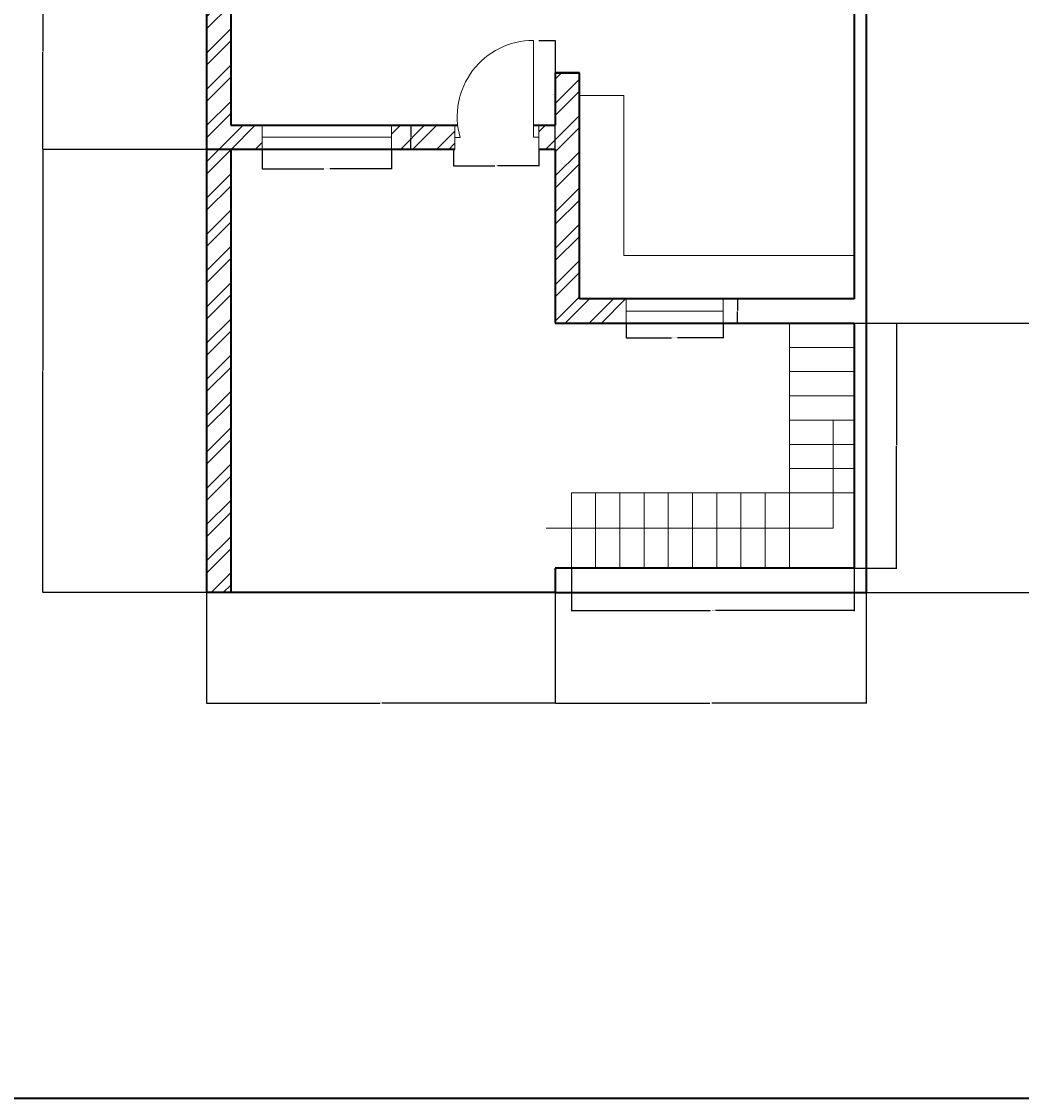
# Model space of a CAD drawing. Units: inches. Extents: x 1850 to 3445, y 1558 to 2756.
# Tile 9 of 13: x 2632 to 3003, y 1558 to 1958. Entities that reach past the tile are written whole.
import ezdxf

# ---------------------------------------------------------------- set-up
doc = ezdxf.new("R2010")
doc.units = ezdxf.units.IN
for name, color, linetype, lineweight in [('A-ANNO-DIMS', 2, 'Continuous', 18), ('A-ANNO-TTLB', 7, 'Continuous', 35), ('A-DOOR', 3, 'Continuous', 18), ('A-FLOR-CASE', 8, 'Continuous', 18), ('A-FLOR-STRS', 7, 'Continuous', 18), ('A-GLAZ', 4, 'Continuous', 18), ('A-WALL', 7, 'Continuous', 35), ('A-WALL-PATT', 252, 'Continuous', 13)]:
    doc.layers.add(name, color=color, linetype=linetype, lineweight=lineweight)
doc.styles.get("Standard").update_dxf_attribs({"font": 'arial.ttf'})
doc.dimstyles.get("Standard").update_dxf_attribs({"dimtxt": 0.18, "dimasz": 0.18, "dimexe": 0.18, "dimexo": 0.0625, "dimgap": 0.09, "dimtad": 0, "dimtih": 1, "dimtoh": 1, "dimdec": 4, "dimzin": 0, "dimdsep": 46, "dimtxsty": 'Standard', "dimcen": 0.09, "dimadec": 0, "dimazin": 0, "dimtfac": 1, "dimtdec": 4, "dimtofl": 0, "dimtmove": 0, "dimatfit": 3, "dimfxl": 1, "dimtolj": 1, "dimtzin": 0, "dimarcsym": 0})

# ---------------------------------------------------------------- blocks, each defined once
blk = doc.blocks.new('WIN-48-W9')
for p, q in [((0, 9), (0, 0)), ((48, 4.5), (48, 9)), ((48, 9), (48, 0)), ((0, 0), (0, 4.5)), ((0, 4.5), (48, 4.5))]:
    blk.add_line(p, q)
blk = doc.blocks.new('WIN-36-W9')
for p, q in [((0, 9), (0, 0)), ((36, 4.5), (36, 9)), ((36, 9), (36, 0)), ((0, 0), (0, 4.5)), ((0, 4.5), (36, 4.5))]:
    blk.add_line(p, q)
blk = doc.blocks.new('DOOR-ENTRY-GROUND')
for p, q in [((29.19, 4.5), (29.19, 40.5)), ((0, 9), (0, 2.33)), ((31.19, 9), (31.19, 0)), ((0, 0), (0, 4.46)), ((0, 4.46), (2, 4.46)), ((31.19, 4.5), (29.19, 4.5)), ((31.19, 0), (31.19, 4.5)), ((0, 2.33), (0, 0))]:
    blk.add_line(p, q)
blk.add_arc((29.19, 12.22), 28.28, 90, 195.9327)
blk = doc.blocks.new('STAIR-L-GROUND')
for p, q in [((81, 28), (81, 91)), ((105, 91), (81, 91)), ((105, 82), (81, 82)), ((105, 73), (81, 73)), ((105, 64), (81, 64)), ((105, 55), (81, 55)), ((105, 46), (81, 46)), ((105, 37), (81, 37)), ((0, 0), (0, 28)), ((0, 28), (105, 28)), ((9, 0), (9, 28)), ((18, 0), (18, 28)), ((27, 0), (27, 28)), ((36, 0), (36, 28)), ((45, 0), (45, 28)), ((54, 0), (54, 28)), ((63, 0), (63, 28)), ((102.7, 28), (72, 28)), ((72, 0), (72, 28)), ((81, 0), (81, 28))]:
    blk.add_line(p, q)
blk = doc.blocks.new('COUNTER-L-GROUND')
for p, q in [((0, 59.33), (16.51, 59.33)), ((16.51, 59.33), (16.51, 0)), ((16.51, 0), (102, 0))]:
    blk.add_line(p, q)
blk = doc.blocks.new('*D34')
at = {"layer": 'A-ANNO-DIMS', "color": 0, "lineweight": -2, "transparency": 16777216}
for p, q in [((2721.5, 1910.15), (2721.5, 1902.84)), ((2769.5, 1910.15), (2769.5, 1902.84)), ((2721.68, 1903.02), (2744.38, 1903.02)), ((2769.32, 1903.02), (2746.62, 1903.02))]:
    blk.add_line(p, q, dxfattribs=at)
at = {"layer": 'A-ANNO-DIMS', "color": 0, "transparency": 16777216}
for points in [[(2721.68, 1903.05), (2721.68, 1902.99), (2721.5, 1903.02)], [(2769.32, 1903.05), (2769.32, 1902.99), (2769.5, 1903.02)]]:
    blk.add_solid(points, dxfattribs=at)
at = {"layer": 'Defpoints', "color": 0, "transparency": 16777216}
for p in [(2721.5, 1910.22), (2769.5, 1910.22), (2769.5, 1903.02)]:
    blk.add_point(p, dxfattribs=at)
at = {"layer": 'A-ANNO-DIMS', "color": 0, "transparency": 16777216, "insert": (2745.5, 1903.02), "char_height": 0.18, "attachment_point": 5}
blk.add_mtext('\\A1;WINDOW 48 TYP.', dxfattribs=at)
blk = doc.blocks.new('*D35')
at = {"layer": 'A-ANNO-DIMS', "color": 0, "lineweight": -2, "transparency": 16777216}
for p, q in [((2769.56, 1919.22), (2776.88, 1919.22)), ((2776.7, 1919.04), (2776.7, 1914.9)), ((2776.7, 1910.4), (2776.7, 1914.54)), ((2769.56, 1910.22), (2776.88, 1910.22))]:
    blk.add_line(p, q, dxfattribs=at)
at = {"layer": 'A-ANNO-DIMS', "color": 0, "transparency": 16777216}
for points in [[(2776.67, 1919.04), (2776.73, 1919.04), (2776.7, 1919.22)], [(2776.67, 1910.4), (2776.73, 1910.4), (2776.7, 1910.22)]]:
    blk.add_solid(points, dxfattribs=at)
at = {"layer": 'Defpoints', "color": 0, "transparency": 16777216}
for p in [(2769.5, 1919.22), (2776.7, 1919.22), (2769.5, 1910.22)]:
    blk.add_point(p, dxfattribs=at)
at = {"layer": 'A-ANNO-DIMS', "color": 0, "transparency": 16777216, "insert": (2776.7, 1914.72), "char_height": 0.18, "attachment_point": 5}
blk.add_mtext('\\A1;9 TYP.', dxfattribs=at)
blk = doc.blocks.new('*D36')
at = {"layer": 'A-ANNO-DIMS', "color": 0, "lineweight": -2, "transparency": 16777216}
for p, q in [((2856.68, 1845.62), (2856.68, 1840.1)), ((2892.68, 1845.62), (2892.68, 1840.1)), ((2856.86, 1840.28), (2873.56, 1840.28)), ((2892.5, 1840.28), (2875.8, 1840.28))]:
    blk.add_line(p, q, dxfattribs=at)
at = {"layer": 'A-ANNO-DIMS', "color": 0, "transparency": 16777216}
for points in [[(2856.86, 1840.31), (2856.86, 1840.25), (2856.68, 1840.28)], [(2892.5, 1840.31), (2892.5, 1840.25), (2892.68, 1840.28)]]:
    blk.add_solid(points, dxfattribs=at)
at = {"layer": 'Defpoints', "color": 0, "transparency": 16777216}
for p in [(2856.68, 1845.68), (2892.68, 1845.68), (2892.68, 1840.28)]:
    blk.add_point(p, dxfattribs=at)
at = {"layer": 'A-ANNO-DIMS', "color": 0, "transparency": 16777216, "insert": (2874.68, 1840.28), "char_height": 0.18, "attachment_point": 5}
blk.add_mtext('\\A1;WINDOW 36 TYP.', dxfattribs=at)
blk = doc.blocks.new('*D37')
at = {"layer": 'A-ANNO-DIMS', "color": 0, "lineweight": -2, "transparency": 16777216}
for p, q in [((2892.74, 1854.68), (2898.26, 1854.68)), ((2898.08, 1854.5), (2898.08, 1850.37)), ((2898.08, 1845.86), (2898.08, 1850)), ((2892.74, 1845.68), (2898.26, 1845.68))]:
    blk.add_line(p, q, dxfattribs=at)
at = {"layer": 'A-ANNO-DIMS', "color": 0, "transparency": 16777216}
for points in [[(2898.05, 1854.5), (2898.11, 1854.5), (2898.08, 1854.68)], [(2898.05, 1845.86), (2898.11, 1845.86), (2898.08, 1845.68)]]:
    blk.add_solid(points, dxfattribs=at)
at = {"layer": 'Defpoints', "color": 0, "transparency": 16777216}
for p in [(2892.68, 1854.68), (2898.08, 1854.68), (2892.68, 1845.68)]:
    blk.add_point(p, dxfattribs=at)
at = {"layer": 'A-ANNO-DIMS', "color": 0, "transparency": 16777216, "insert": (2898.08, 1850.18), "char_height": 0.18, "attachment_point": 5}
blk.add_mtext('\\A1;9 TYP.', dxfattribs=at)
blk = doc.blocks.new('*D60')
at = {"layer": 'A-ANNO-DIMS', "color": 0, "lineweight": -2, "transparency": 16777216}
for p, q in [((2824.3, 1950.72), (2830.49, 1950.72)), ((2830.31, 1950.54), (2830.31, 1930.65)), ((2830.31, 1910.4), (2830.31, 1930.28)), ((2824.3, 1910.22), (2830.49, 1910.22))]:
    blk.add_line(p, q, dxfattribs=at)
at = {"layer": 'A-ANNO-DIMS', "color": 0, "transparency": 16777216}
for points in [[(2830.28, 1950.54), (2830.34, 1950.54), (2830.31, 1950.72)], [(2830.28, 1910.4), (2830.34, 1910.4), (2830.31, 1910.22)]]:
    blk.add_solid(points, dxfattribs=at)
at = {"layer": 'Defpoints', "color": 0, "transparency": 16777216}
for p in [(2824.24, 1950.72), (2830.31, 1950.72), (2824.24, 1910.22)]:
    blk.add_point(p, dxfattribs=at)
at = {"layer": 'A-ANNO-DIMS', "color": 0, "transparency": 16777216, "insert": (2830.31, 1930.47), "char_height": 0.18, "attachment_point": 5}
blk.add_mtext('\\A1;ENTRY DOOR 41 TYP.', dxfattribs=at)
blk = doc.blocks.new('*D61')
at = {"layer": 'A-ANNO-DIMS', "color": 0, "lineweight": -2, "transparency": 16777216}
for p, q in [((2792.61, 1910.15), (2792.61, 1903.96)), ((2824.24, 1910.15), (2824.24, 1903.96)), ((2792.79, 1904.14), (2807.9, 1904.14)), ((2824.06, 1904.14), (2808.95, 1904.14))]:
    blk.add_line(p, q, dxfattribs=at)
at = {"layer": 'A-ANNO-DIMS', "color": 0, "transparency": 16777216}
for points in [[(2792.79, 1904.17), (2792.79, 1904.11), (2792.61, 1904.14)], [(2824.06, 1904.17), (2824.06, 1904.11), (2824.24, 1904.14)]]:
    blk.add_solid(points, dxfattribs=at)
at = {"layer": 'Defpoints', "color": 0, "transparency": 16777216}
for p in [(2792.61, 1910.22), (2824.24, 1910.22), (2824.24, 1904.14)]:
    blk.add_point(p, dxfattribs=at)
at = {"layer": 'A-ANNO-DIMS', "color": 0, "transparency": 16777216, "insert": (2808.42, 1904.14), "char_height": 0.18, "attachment_point": 5}
blk.add_mtext('\\A1;32 TYP.', dxfattribs=at)
blk = doc.blocks.new('*D68')
at = {"layer": 'A-ANNO-DIMS', "color": 0, "lineweight": -2, "transparency": 16777216}
for p, q in [((2836.32, 1754.62), (2836.32, 1738.75)), ((2941.32, 1754.62), (2941.32, 1738.75)), ((2836.5, 1738.93), (2887.82, 1738.93)), ((2941.14, 1738.93), (2889.82, 1738.93))]:
    blk.add_line(p, q, dxfattribs=at)
at = {"layer": 'A-ANNO-DIMS', "color": 0, "transparency": 16777216}
for points in [[(2836.5, 1738.96), (2836.5, 1738.9), (2836.32, 1738.93)], [(2941.14, 1738.96), (2941.14, 1738.9), (2941.32, 1738.93)]]:
    blk.add_solid(points, dxfattribs=at)
at = {"layer": 'Defpoints', "color": 0, "transparency": 16777216}
for p in [(2836.32, 1754.68), (2941.32, 1754.68), (2941.32, 1738.93)]:
    blk.add_point(p, dxfattribs=at)
at = {"layer": 'A-ANNO-DIMS', "color": 0, "transparency": 16777216, "insert": (2888.82, 1738.93), "char_height": 0.18, "attachment_point": 5}
blk.add_mtext('\\A1;STAIR 105 TYP.', dxfattribs=at)
blk = doc.blocks.new('*D69')
at = {"layer": 'A-ANNO-DIMS', "color": 0, "lineweight": -2, "transparency": 16777216}
for p, q in [((2941.38, 1845.68), (2957.25, 1845.68)), ((2957.07, 1845.5), (2957.07, 1800.37)), ((2957.07, 1754.86), (2957.07, 1800)), ((2941.38, 1754.68), (2957.25, 1754.68))]:
    blk.add_line(p, q, dxfattribs=at)
at = {"layer": 'A-ANNO-DIMS', "color": 0, "transparency": 16777216}
for points in [[(2957.04, 1845.5), (2957.1, 1845.5), (2957.07, 1845.68)], [(2957.04, 1754.86), (2957.1, 1754.86), (2957.07, 1754.68)]]:
    blk.add_solid(points, dxfattribs=at)
at = {"layer": 'Defpoints', "color": 0, "transparency": 16777216}
for p in [(2941.32, 1845.68), (2957.07, 1845.68), (2941.32, 1754.68)]:
    blk.add_point(p, dxfattribs=at)
at = {"layer": 'A-ANNO-DIMS', "color": 0, "transparency": 16777216, "insert": (2957.07, 1800.18), "char_height": 0.18, "attachment_point": 5}
blk.add_mtext('\\A1;91 TYP.', dxfattribs=at)
blk = doc.blocks.new('*D92')
at = {"layer": 'A-ANNO-DIMS', "color": 0, "lineweight": -2, "transparency": 16777216}
for p, q in [((2700.82, 1745.62), (2700.82, 1704.45)), ((2830.32, 1745.62), (2830.32, 1704.45)), ((2701, 1704.63), (2765.19, 1704.63)), ((2830.14, 1704.63), (2765.96, 1704.63))]:
    blk.add_line(p, q, dxfattribs=at)
at = {"layer": 'A-ANNO-DIMS', "color": 0, "transparency": 16777216}
for points in [[(2701, 1704.66), (2701, 1704.6), (2700.82, 1704.63)], [(2830.14, 1704.66), (2830.14, 1704.6), (2830.32, 1704.63)]]:
    blk.add_solid(points, dxfattribs=at)
at = {"layer": 'Defpoints', "color": 0, "transparency": 16777216}
for p in [(2700.82, 1745.68), (2830.32, 1745.68), (2830.32, 1704.63)]:
    blk.add_point(p, dxfattribs=at)
at = {"layer": 'A-ANNO-DIMS', "color": 0, "transparency": 16777216, "insert": (2765.57, 1704.63), "char_height": 0.18, "attachment_point": 5}
blk.add_mtext('\\A1;129.5', dxfattribs=at)
blk = doc.blocks.new('*D93')
at = {"layer": 'A-ANNO-DIMS', "color": 0, "lineweight": -2, "transparency": 16777216}
for p, q in [((2830.32, 1745.62), (2830.32, 1704.45)), ((2945.82, 1745.62), (2945.82, 1704.45)), ((2830.5, 1704.63), (2887.69, 1704.63)), ((2945.64, 1704.63), (2888.46, 1704.63))]:
    blk.add_line(p, q, dxfattribs=at)
at = {"layer": 'A-ANNO-DIMS', "color": 0, "transparency": 16777216}
for points in [[(2830.5, 1704.66), (2830.5, 1704.6), (2830.32, 1704.63)], [(2945.64, 1704.66), (2945.64, 1704.6), (2945.82, 1704.63)]]:
    blk.add_solid(points, dxfattribs=at)
at = {"layer": 'Defpoints', "color": 0, "transparency": 16777216}
for p in [(2830.32, 1745.68), (2945.82, 1745.68), (2945.82, 1704.63)]:
    blk.add_point(p, dxfattribs=at)
at = {"layer": 'A-ANNO-DIMS', "color": 0, "transparency": 16777216, "insert": (2888.07, 1704.63), "char_height": 0.18, "attachment_point": 5}
blk.add_mtext('\\A1;115.5', dxfattribs=at)
blk = doc.blocks.new('*D97')
at = {"layer": 'A-ANNO-DIMS', "color": 0, "lineweight": -2, "transparency": 16777216}
for p, q in [((2700.76, 1910.22), (2639.89, 1910.22)), ((2640.07, 1910.04), (2640.07, 1828.13)), ((2640.07, 1745.86), (2640.07, 1827.77)), ((2700.76, 1745.68), (2639.89, 1745.68))]:
    blk.add_line(p, q, dxfattribs=at)
at = {"layer": 'A-ANNO-DIMS', "color": 0, "transparency": 16777216}
for points in [[(2640.04, 1910.04), (2640.1, 1910.04), (2640.07, 1910.22)], [(2640.04, 1745.86), (2640.1, 1745.86), (2640.07, 1745.68)]]:
    blk.add_solid(points, dxfattribs=at)
at = {"layer": 'Defpoints', "color": 0, "transparency": 16777216}
for p in [(2640.07, 1910.22), (2700.82, 1910.22), (2700.82, 1745.68)]:
    blk.add_point(p, dxfattribs=at)
at = {"layer": 'A-ANNO-DIMS', "color": 0, "transparency": 16777216, "insert": (2640.07, 1827.95), "char_height": 0.18, "attachment_point": 5}
blk.add_mtext('\\A1;164.53', dxfattribs=at)
blk = doc.blocks.new('*D98')
at = {"layer": 'A-ANNO-DIMS', "color": 0, "lineweight": -2, "transparency": 16777216}
for p, q in [((2700.76, 1982.85), (2639.89, 1982.85)), ((2640.07, 1982.67), (2640.07, 1946.71)), ((2640.07, 1910.4), (2640.07, 1946.35)), ((2700.76, 1910.22), (2639.89, 1910.22))]:
    blk.add_line(p, q, dxfattribs=at)
at = {"layer": 'A-ANNO-DIMS', "color": 0, "transparency": 16777216}
for points in [[(2640.04, 1982.67), (2640.1, 1982.67), (2640.07, 1982.85)], [(2640.04, 1910.4), (2640.1, 1910.4), (2640.07, 1910.22)]]:
    blk.add_solid(points, dxfattribs=at)
at = {"layer": 'Defpoints', "color": 0, "transparency": 16777216}
for p in [(2640.07, 1982.85), (2700.82, 1982.85), (2700.82, 1910.22)]:
    blk.add_point(p, dxfattribs=at)
at = {"layer": 'A-ANNO-DIMS', "color": 0, "transparency": 16777216, "insert": (2640.07, 1946.53), "char_height": 0.18, "attachment_point": 5}
blk.add_mtext('\\A1;72.63', dxfattribs=at)
blk = doc.blocks.new('*D102')
at = {"layer": 'A-ANNO-DIMS', "color": 0, "lineweight": -2, "transparency": 16777216}
for p, q in [((2941.38, 1845.68), (3346.97, 1845.68)), ((3346.79, 1845.5), (3346.79, 1795.87)), ((3346.79, 1745.86), (3346.79, 1795.5)), ((2945.88, 1745.68), (3346.97, 1745.68))]:
    blk.add_line(p, q, dxfattribs=at)
at = {"layer": 'A-ANNO-DIMS', "color": 0, "transparency": 16777216}
for points in [[(3346.76, 1845.5), (3346.82, 1845.5), (3346.79, 1845.68)], [(3346.76, 1745.86), (3346.82, 1745.86), (3346.79, 1745.68)]]:
    blk.add_solid(points, dxfattribs=at)
at = {"layer": 'Defpoints', "color": 0, "transparency": 16777216}
for p in [(2941.32, 1845.68), (3346.79, 1845.68), (2945.82, 1745.68)]:
    blk.add_point(p, dxfattribs=at)
at = {"layer": 'A-ANNO-DIMS', "color": 0, "transparency": 16777216, "insert": (3346.79, 1795.68), "char_height": 0.18, "attachment_point": 5}
blk.add_mtext('\\A1;100', dxfattribs=at)

msp = doc.modelspace()

# ---------------------------------------------------------------- hatches: boundary and pattern name
at = {"layer": 'A-WALL-PATT'}
h = msp.add_hatch(dxfattribs=at)
h.set_pattern_fill('ANSI32', color=256)
h.set_pattern_definition([(45, (660.551, 0), (-6.735192, 6.735192), []), (45, (665.041, 0), (-6.735192, 6.735192), [])])
h.paths.add_polyline_path([(3180.1061, 1907.3936), (3184.5492, 1907.3936), (3184.5492, 1916.3936), (3180.1061, 1916.3936), (3175.6061, 1916.3936), (3171.1061, 1916.3936), (3171.1061, 1907.3936), (3175.6061, 1907.3936), (3175.6061, 1742.1843), (3175.6061, 1737.6843), (3256.6061, 1737.6843), (3256.6061, 1976.4962), (3252.1061, 1976.4962), (3252.1061, 1916.3936), (3221.8172, 1916.3936), (3221.8172, 1907.3936), (3252.1061, 1907.3936), (3252.1061, 1746.6843), (3180.1061, 1746.6843)])
h.paths.add_polyline_path([(2737.1986, 2211.6843), (2737.1986, 2216.1843), (2700.822, 2216.1843), (2700.822, 2175.83), (2705.322, 2175.83), (2709.822, 2175.83), (2709.822, 2207.1843), (2737.1986, 2207.1843)])
h.paths.add_polyline_path([(2872.322, 2216.1843), (2797.1986, 2216.1843), (2797.1986, 2207.1843), (2872.322, 2207.1843)])
h.paths.add_polyline_path([(2945.822, 2154.1843), (2911.1674, 2154.1843), (2911.1674, 2149.6843), (2941.322, 2149.6843), (2941.322, 2075.1843), (2896.9138, 2075.1843), (2896.9138, 2070.6843), (2945.822, 2070.6843)])
h.paths.add_polyline_path([(2888.8991, 2154.1843), (2867.822, 2154.1843), (2867.822, 2075.1843), (2862.5325, 2075.1843), (2862.5325, 2070.6843), (2876.0169, 2070.6843), (2876.0169, 2072.9343), (2876.0169, 2075.1843), (2872.322, 2075.1843), (2872.322, 2149.6843), (2888.8991, 2149.6843)])
h.paths.add_polyline_path([(2709.822, 2115.83), (2700.822, 2115.83), (2700.822, 2042.8465), (2709.822, 2042.8465), (2709.822, 2070.6843), (2829.1562, 2070.6843), (2829.1562, 2072.9343), (2829.1562, 2075.1843), (2709.822, 2075.1843)])
h.paths.add_polyline_path([(2709.822, 1982.8465), (2700.822, 1982.8465), (2700.822, 1910.2175), (2721.4986, 1910.2175), (2721.4986, 1914.7175), (2721.4986, 1919.2175), (2709.822, 1919.2175)])
h.paths.add_polyline_path([(2793.0443, 1919.2175), (2769.4986, 1919.2175), (2769.4986, 1910.2175), (2793.0443, 1910.2175), (2793.0443, 1914.6749)])
h.paths.add_polyline_path([(2839.322, 1938.6843), (2830.322, 1938.6843), (2830.322, 1919.2175), (2824.2376, 1919.2175), (2824.2376, 1910.2175), (2830.322, 1910.2175), (2830.322, 1854.6843), (2830.322, 1845.6843), (2856.6792, 1845.6843), (2856.6792, 1850.1843), (2856.6792, 1854.6843), (2839.322, 1854.6843)])
h.paths.add_polyline_path([(2709.822, 1910.2175), (2700.822, 1910.2175), (2700.822, 1745.6843), (2709.822, 1745.6843)])
h.paths.add_polyline_path([(2807.4367, 1766.7204), (2819.64, 1766.7204), (2819.64, 1777.0239), (2807.4367, 1777.0239)], flags=9)
h.paths.add_polyline_path([(2844.0169, 1798.4016), (2887.2843, 1798.4016), (2887.2843, 1817.0589), (2844.0169, 1817.0589)], flags=9)
h.paths.add_polyline_path([(2731.4135, 1867.537), (2770.5302, 1867.537), (2770.5302, 1886.1943), (2731.4135, 1886.1943)], flags=9)

# ---------------------------------------------------------------- linework, layer by layer
at = {"layer": 'A-ANNO-TTLB'}
msp.add_lwpolyline([(1850.1793, 2756.3177), (3445.2682, 2756.3177), (3445.2682, 1557.7728), (1850.1793, 1557.7728)], close=True, dxfattribs=at)
at = {"layer": 'A-FLOR-STRS'}
for p, q in [((2933.491, 1769.5741), (2933.491, 1809.6843)), ((2827.0025, 1769.5741), (2933.491, 1769.5741))]:
    msp.add_line(p, q, dxfattribs=at)
at = {"layer": 'A-WALL'}
for p, q in [((2700.822, 2216.1843), (2700.822, 1745.6843)), ((2945.822, 2207.1843), (2945.822, 1745.6843)), ((2709.822, 2070.6843), (2709.822, 1919.2175)), ((2941.322, 2070.6843), (2941.322, 1854.6843)), ((2830.322, 1938.6843), (2839.322, 1938.6843)), ((2839.322, 1938.6843), (2830.322, 1938.6843)), ((2830.322, 1938.6843), (2830.322, 1919.2175)), ((2839.322, 1854.6843), (2839.322, 1938.6843)), ((2709.822, 1919.2175), (2794.1419, 1919.2175)), ((2822.2376, 1919.2175), (2830.322, 1919.2175)), ((2793.0443, 1910.2175), (2700.822, 1910.2175)), ((2709.822, 1910.2175), (2709.822, 1745.6843)), ((2830.322, 1910.2175), (2824.2376, 1910.2175)), ((2830.322, 1910.2175), (2830.322, 1854.6843)), ((2830.322, 1854.6843), (2830.322, 1845.6843)), ((2941.322, 1854.6843), (2839.322, 1854.6843)), ((2830.322, 1845.6843), (2941.322, 1845.6843)), ((2941.322, 1845.6843), (2941.322, 1754.6843)), ((2941.322, 1845.6843), (2941.322, 1754.6843)), ((2941.322, 1754.6843), (2830.322, 1754.6843)), ((2830.322, 1754.6843), (2830.322, 1745.6843)), ((2830.322, 1745.6843), (2700.822, 1745.6843)), ((2830.322, 1745.6843), (2941.322, 1745.6843)), ((2941.322, 1745.6843), (2945.822, 1745.6843))]:
    msp.add_line(p, q, dxfattribs=at)

# ---------------------------------------------------------------- block references
at = {"layer": 'A-DOOR'}
msp.add_blockref('DOOR-ENTRY-GROUND', (2793.0445, 1910.217), dxfattribs=at)
at = {"layer": 'A-FLOR-CASE'}
msp.add_blockref('COUNTER-L-GROUND', (2839.3215, 1870.864), dxfattribs=at)
at = {"layer": 'A-FLOR-STRS'}
msp.add_blockref('STAIR-L-GROUND', (2836.3215, 1754.684), dxfattribs=at)
at = {"layer": 'A-GLAZ'}
for name, p in [('WIN-48-W9', (2721.4985, 1910.217)), ('WIN-36-W9', (2856.6795, 1845.684))]:
    msp.add_blockref(name, p, dxfattribs=at)

# ---------------------------------------------------------------- dimensions: what is measured, and where the dimension line sits
at = {"layer": 'A-ANNO-DIMS'}
for base, p1, p2, override, picture, middle in [((2640.0656, 1982.8465), (2700.822, 1910.2175), (2700.822, 1982.8465), {"dimdec": 2, "dimlfac": 1, "dimrnd": 0, "dimzin": 0, "dimdsep": 46, "dimlunit": 2}, '*D98', (2640.0656, 1946.532)), ((2640.0656, 1910.2175), (2700.822, 1745.6843), (2700.822, 1910.2175), {"dimdec": 2, "dimlfac": 1, "dimrnd": 0, "dimzin": 0, "dimdsep": 46, "dimlunit": 2}, '*D97', (2640.0656, 1827.9509)), ((3346.7887, 1845.6843), (2945.822, 1745.6843), (2941.322, 1845.6843), {"dimdec": 0, "dimlfac": 1, "dimrnd": 0, "dimzin": 0, "dimdsep": 46, "dimlunit": 2}, '*D102', (3346.7887, 1795.6843))]:
    dim = msp.add_linear_dim(base=base, p1=p1, p2=p2, angle=90, dimstyle='Standard', override=override, dxfattribs=at)
    dim.commit()
    dim.dimension.update_dxf_attribs({"geometry": picture, "text_midpoint": middle})
for base, p1, p2, text, picture, middle in [((2830.3125694243, 1950.7174566172), (2824.2375694243, 1910.2174566172), (2824.2375694243, 1950.7174566172), 'ENTRY DOOR <> TYP.', '*D60', (2830.3125694243, 1930.4674566172)), ((2776.6986, 1919.2175), (2769.4986, 1910.2175), (2769.4986, 1919.2175), '<> TYP.', '*D35', (2776.6986, 1914.7175)), ((2898.0792, 1854.6843), (2892.6792, 1845.6843), (2892.6792, 1854.6843), '<> TYP.', '*D37', (2898.0792, 1850.1843)), ((2957.072, 1845.6843), (2941.322, 1754.6843), (2941.322, 1845.6843), '<> TYP.', '*D69', (2957.072, 1800.1843))]:
    dim = msp.add_linear_dim(base=base, p1=p1, p2=p2, angle=90, text=text, dimstyle='Standard', override={"dimdec": 0, "dimlfac": 1, "dimrnd": 0, "dimzin": 0, "dimdsep": 46, "dimlunit": 2}, dxfattribs=at)
    dim.commit()
    dim.dimension.update_dxf_attribs({"geometry": picture, "text_midpoint": middle})
for base, p1, p2, text, picture, middle in [((2769.4986, 1903.0175), (2721.4986, 1910.2175), (2769.4986, 1910.2175), 'WINDOW <> TYP.', '*D34', (2745.4986, 1903.0175)), ((2824.2376, 1904.1425), (2792.6087, 1910.2175), (2824.2376, 1910.2175), '<> TYP.', '*D61', (2808.4231, 1904.1425)), ((2892.6792, 1840.2843), (2856.6792, 1845.6843), (2892.6792, 1845.6843), 'WINDOW <> TYP.', '*D36', (2874.6792, 1840.2843)), ((2941.322, 1738.9343), (2836.322, 1754.6843), (2941.322, 1754.6843), 'STAIR <> TYP.', '*D68', (2888.822, 1738.9343))]:
    dim = msp.add_linear_dim(base=base, p1=p1, p2=p2, text=text, dimstyle='Standard', override={"dimdec": 0, "dimlfac": 1, "dimrnd": 0, "dimzin": 0, "dimdsep": 46, "dimlunit": 2}, dxfattribs=at)
    dim.commit()
    dim.dimension.update_dxf_attribs({"geometry": picture, "text_midpoint": middle})
for base, p1, p2, picture, middle in [((2830.322, 1704.6343), (2700.822, 1745.6843), (2830.322, 1745.6843), '*D92', (2765.572, 1704.6343)), ((2945.822, 1704.6343), (2830.322, 1745.6843), (2945.822, 1745.6843), '*D93', (2888.072, 1704.6343))]:
    dim = msp.add_linear_dim(base=base, p1=p1, p2=p2, dimstyle='Standard', override={"dimdec": 1, "dimlfac": 1, "dimrnd": 0, "dimzin": 0, "dimdsep": 46, "dimlunit": 2}, dxfattribs=at)
    dim.commit()
    dim.dimension.update_dxf_attribs({"geometry": picture, "text_midpoint": middle})

doc.saveas('drawing.dxf')
